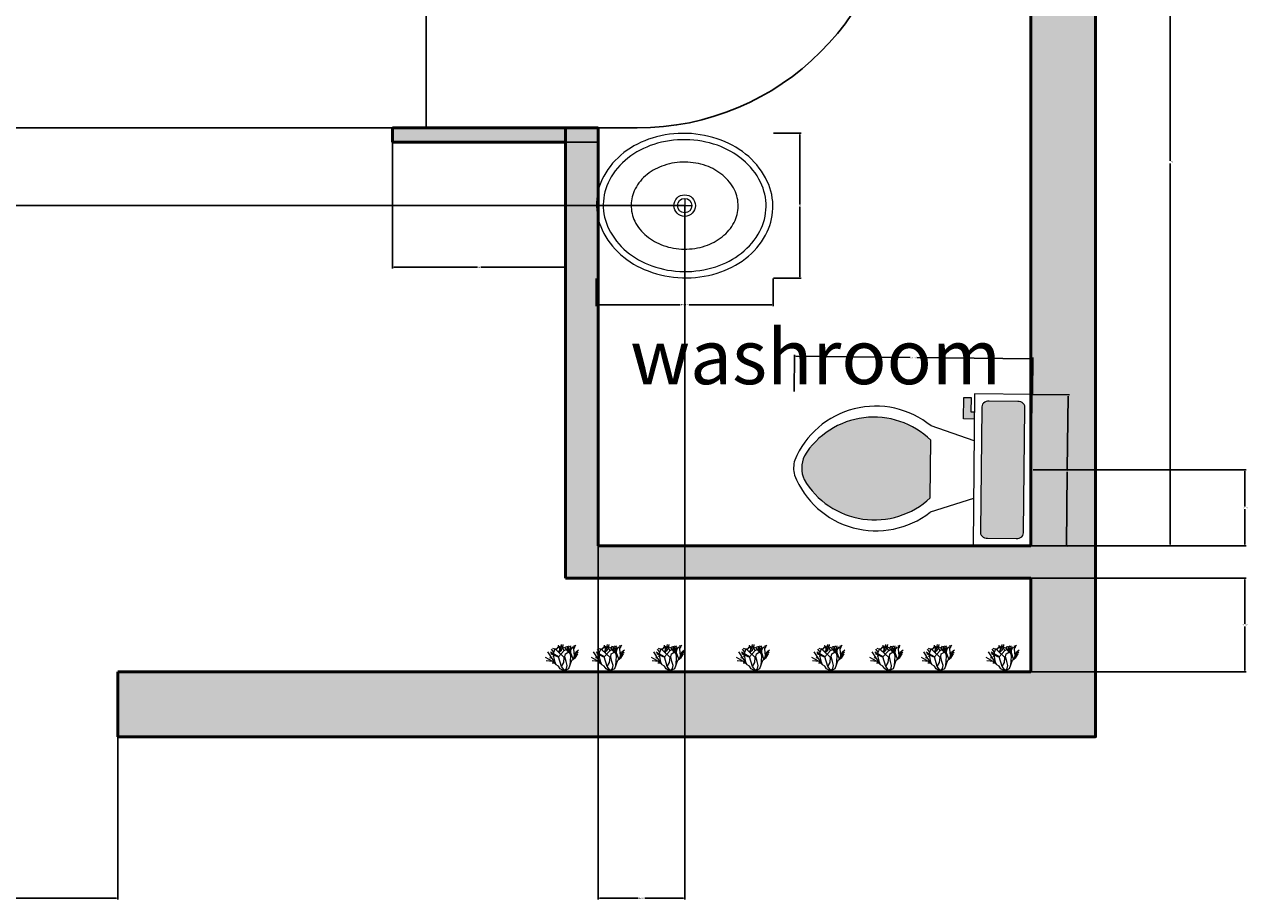
# Model space of a CAD drawing. Units: inches. Extents: x 2578 to 2919, y 51 to 451.
# Tile 3 of 5: x 2750 to 2919, y 51 to 172. Entities that reach past the tile are written whole.
import ezdxf

# ---------------------------------------------------------------- set-up
doc = ezdxf.new("R2010")
doc.units = ezdxf.units.IN
for name, color, linetype, lineweight in [('A-ANNO-DIMS', 2, 'Continuous', 18), ('A-AREA-IDEN', 7, 'Continuous', 25), ('A-DOOR', 4, 'Continuous', 25), ('A-FLOR-FIXT', 9, 'Continuous', 18), ('A-FURN-PATT', 253, 'Continuous', 13), ('A-WALL', 7, 'Continuous', 50), ('A-WALL-PATT', 250, 'Continuous', 13), ('L-PLNT', 94, 'Continuous', 13)]:
    doc.layers.add(name, color=color, linetype=linetype, lineweight=lineweight)
doc.layers.add('A-DOOR-PATT', color=29, linetype='Continuous', lineweight=13, true_color=0x4f342a)
doc.styles.get("Standard").update_dxf_attribs({"font": 'arial.ttf'})
doc.dimstyles.get("Standard").update_dxf_attribs({"dimtxt": 0.18, "dimasz": 0.18, "dimexe": 0.18, "dimexo": 0.0625, "dimgap": 0.09, "dimtad": 0, "dimtih": 1, "dimtoh": 1, "dimdec": 4, "dimzin": 0, "dimdsep": 46, "dimtxsty": 'Standard', "dimcen": 0.09, "dimadec": 0, "dimazin": 0, "dimtfac": 1, "dimtdec": 4, "dimtofl": 0, "dimtmove": 0, "dimatfit": 3, "dimfxl": 1, "dimtolj": 1, "dimtzin": 0, "dimarcsym": 0})

# ---------------------------------------------------------------- blocks, each defined once
blk = doc.blocks.new('*U3')
for p, q in [((0, 0), (0, -6)), ((40, 0), (40, -6))]:
    blk.add_line(p, q)
blk.add_lwpolyline([(0, 0), (0, 40), (1.75, 40), (1.75, 0)], close=True)
blk.add_arc((0, 0), 40, 0, 90)
blk = doc.blocks.new('Toilet - top')
for p, q in [((9.5, -6), (9.5, -2)), ((-8, -8.5), (-8, -8)), ((-7, -8), (-7, -9.5)), ((-4, -8), (-6, -14)), ((4, -8), (6, -14)), ((-10, -8.5), (-8, -8.5)), ((-10, -9.5), (-10, -8.5)), ((-7, -9.5), (-10, -9.5)), ((4, -14), (-4, -14))]:
    blk.add_line(p, q)
blk.add_lwpolyline([(10.5, -8), (10.5, 0), (-10.5, 0), (-10.5, -8)], close=True)
for points in [[(8.5, -1), (-8.5, -1)], [(-9.5, -2), (-9.5, -6)], [(-8.5, -7), (8.5, -7)]]:
    blk.add_lwpolyline(points)
for centre, radius, start, end in [((-8.62, -1.88), 0.884, 81.8699, 188.1301), ((8.62, -1.88), 0.884, 351.8699, 98.1301), ((-8.62, -6.12), 0.884, 171.8699, 278.1301), ((8.62, -6.12), 0.884, 261.8699, 8.1301), ((3.52, -21.58), 12.17, 141.4691, 247.9714), ((4.2, -21.82), 11.33, 136.3677, 238.9468), ((-3.52, -21.58), 12.17, 292.0284, 38.5307), ((-4.2, -21.82), 11.33, 301.053, 43.6321), ((0, -27.88), 4, 245.7318, 294.2682), ((0, -29), 4, 254.8605, 285.1395)]:
    blk.add_arc(centre, radius, start, end)
blk = doc.blocks.new('Sink - Oval top')
for p, q in [((-1, 0), (1, 0)), ((0, 1), (0, -1))]:
    blk.add_line(p, q)
for points in [[(-12.23, 0.39, 0.117634), (-11.46, -3.36, 0.104469), (-8.88, -6.8, 0.090016), (-5.08, -9.07, 0.08192), (-0.32, -10.02, 0.08192), (4.49, -9.38, 0.090016), (8.42, -7.36, 0.104469), (11.22, -4.09, 0.117634), (12.23, -0.39, 0.117634), (11.46, 3.36, 0.104469), (8.88, 6.8, 0.090016), (5.08, 9.07, 0.08192), (0.32, 10.02, 0.08192), (-4.49, 9.38, 0.090016), (-8.42, 7.36, 0.104469), (-11.22, 4.09, 0.117634)], [(-11.29, 0.16, 0.118622), (-10.52, -3.25, 0.104678), (-8.07, -6.36, 0.089562), (-4.54, -8.37, 0.081185), (-0.13, -9.15, 0.081185), (4.3, -8.49, 0.089562), (7.89, -6.58, 0.104678), (10.42, -3.55, 0.118622), (11.29, -0.16, 0.118622), (10.52, 3.25, 0.104678), (8.07, 6.36, 0.089562), (4.54, 8.37, 0.081185), (0.13, 9.15, 0.081185), (-4.3, 8.49, 0.089562), (-7.89, 6.58, 0.104678), (-10.42, 3.55, 0.118622)], [(-7.42, 0.08, 0.118283), (-6.91, -2.17, 0.104607), (-5.29, -4.21, 0.089718), (-2.97, -5.53, 0.081436), (-0.07, -6.04, 0.081436), (2.84, -5.59, 0.089718), (5.2, -4.33, 0.104607), (6.86, -2.32, 0.118283), (7.42, -0.08, 0.118283), (6.91, 2.17, 0.104607), (5.29, 4.21, 0.089718), (2.97, 5.53, 0.081436), (0.07, 6.04, 0.081436), (-2.84, 5.59, 0.089718), (-5.2, 4.33, 0.104607), (-6.86, 2.32, 0.118283)]]:
    blk.add_lwpolyline(points, format="xyb", close=True)
for radius in [1.5, 1]:
    blk.add_circle((0, 0), radius)
blk = doc.blocks.new('*U11')
for p, q in [((-14.88, 18.24), (-12.96, 20.64)), ((-12.471, 19.775), (-12.898, 22.044)), ((-11.28, 19.619), (-12.104, 21.184)), ((-11.921, 18.836), (-10.64, 20.401)), ((-11.433, 18.289), (-10.457, 22.749)), ((-8.16, 17.76), (-10.56, 21.6)), ((-9.48, 19.775), (-8.992, 22.592)), ((-7.2, 19.68), (-6.24, 21.12)), ((-5.086, 17.741), (-5.513, 21.34)), ((-5.28, 19.2), (-3.84, 21.6)), ((-3.84, 16.8), (-0.96, 20.64)), ((-3.377, 18.602), (-2.888, 21.575)), ((-0.508, 21.888), (-0.081, 20.558)), ((-0.203, 19.149), (0.102, 21.34)), ((-0.142, 19.384), (0.59, 20.401)), ((-0.02, 20.01), (0.896, 21.105)), ((0.041, 20.714), (1.384, 22.044)), ((0.102, 21.34), (0.835, 21.888)), ((-17.76, 8.64), (-23.663, 11.961)), ((-18.24, 11.04), (-21.755, 16.655)), ((-18.24, 11.04), (-20.16, 11.52)), ((-12.96, 12.48), (-19.68, 16.32)), ((-13.92, 12.48), (-19.2, 14.88)), ((-16.8, 16.32), (-18.72, 18.72)), ((-15.84, 8.16), (-18.24, 11.04)), ((-14.88, 18.24), (-17.76, 19.2)), ((-16.8, 12.48), (-17.76, 12.96)), ((-16.8, 16.32), (-15.36, 19.68)), ((-16.8, 12.48), (-16.8, 16.32)), ((-15.84, 8.16), (-16.8, 12.48)), ((-8.16, 12), (-14.88, 18.24)), ((-12.96, 12.48), (-13.92, 12.48)), ((-13.325, 16.724), (-11.433, 18.289)), ((-12.96, 12.48), (-8.16, 17.76)), ((-10.56, 4.32), (-12.96, 12.48)), ((-11.677, 19.071), (-12.471, 19.775)), ((-12.043, 15.628), (-11.921, 18.836)), ((-11.982, 16.802), (-10.579, 18.054)), ((-10.579, 18.054), (-9.846, 19.697)), ((-7.2, 19.68), (-8.64, 20.16)), ((-8.64, 7.68), (-8.16, 12)), ((-8.16, 17.76), (-5.28, 19.2)), ((-7.68, 12.48), (-7.2, 14.88)), ((-6.72, 8.64), (-7.68, 12.48)), ((-4.8, 16.32), (-7.2, 19.68)), ((-7.2, 14.88), (-3.84, 16.8)), ((-3.377, 15.315), (-5.086, 17.819)), ((-2.88, 12.96), (-4.32, 19.68)), ((-2.766, 16.802), (-3.377, 18.602)), ((-3.36, 5.28), (-2.88, 12.96)), ((-2.88, 15.84), (-2.4, 20.16)), ((-0.96, 10.56), (-2.88, 15.84)), ((-1.92, 9.6), (0.96, 12)), ((-0.48, 10.8), (0.346, 13.203)), ((0.346, 13.203), (-0.203, 19.149)), ((0.346, 13.203), (1.323, 16.254)), ((0.96, 12), (1.44, 15.36)), ((0.96, 12), (2.88, 14.88)), ((1.323, 16.254), (3.642, 18.289)), ((1.44, 15.36), (2.88, 17.28)), ((1.92, 13.44), (2.4, 15.36)), ((2.4, 15.36), (3.36, 16.32)), ((-17.76, 8.64), (-23.128, 9.222)), ((-16.32, 7.2), (-18.24, 7.2)), ((-14.88, 5.76), (-17.76, 8.64)), ((-15.84, 0.48), (-17.76, 0)), ((-14.88, 5.76), (-15.84, 8.16)), ((-13.44, 0.48), (-15.84, 0.48)), ((-12.96, 4.8), (-14.88, 5.76)), ((-9.6, 0.96), (-13.44, 0.48)), ((-11.52, 2.4), (-12.96, 4.8)), ((-9.6, 0.96), (-12.96, 0)), ((-8.64, 0.96), (-11.52, 2.4)), ((-10.56, 4.32), (-8.64, 7.68)), ((-8.64, 1.92), (-10.56, 4.32)), ((-9.6, 0.96), (-7.68, 0.96)), ((-8.64, 0.96), (-4.32, 2.88)), ((-8.64, 0.96), (-6.24, 2.88)), ((-8.64, 0.96), (-8.64, 1.92)), ((-8.64, 0.96), (-2.88, 0.96)), ((-7.68, 0.96), (-6.24, 0.48)), ((-5.76, 5.28), (-6.72, 8.64)), ((-6.24, 2.88), (-5.76, 5.28)), ((-6.24, 0.48), (-3.36, 0)), ((-4.32, 2.88), (-1.92, 9.6)), ((-2.88, 0.96), (0, 0))]:
    blk.add_line(p, q)
blk = doc.blocks.new('*D21')
at = {"layer": 'A-ANNO-DIMS', "color": 0, "lineweight": -2, "transparency": 16777216}
for p, q in [((2856.36, 121.01), (2856.42, 126.09)), ((2856.59, 125.9), (2872.47, 125.74)), ((2889.28, 125.56), (2873.4, 125.73)), ((2889.41, 120.66), (2889.46, 125.73))]:
    blk.add_line(p, q, dxfattribs=at)
at = {"layer": 'A-ANNO-DIMS', "color": 0, "transparency": 16777216}
for points in [[(2856.59, 125.93), (2856.59, 125.87), (2856.41, 125.91)], [(2889.28, 125.59), (2889.28, 125.53), (2889.46, 125.55)]]:
    blk.add_solid(points, dxfattribs=at)
at = {"layer": 'Defpoints', "color": 0, "transparency": 16777216}
for p in [(2889.46, 125.55), (2856.36, 120.95), (2889.41, 120.6)]:
    blk.add_point(p, dxfattribs=at)
at = {"layer": 'A-ANNO-DIMS', "color": 0, "transparency": 16777216, "insert": (2872.94, 125.73), "char_height": 0.18, "attachment_point": 5}
blk.add_mtext('\\A1;WC 33', dxfattribs=at)
blk = doc.blocks.new('*D22')
at = {"layer": 'A-ANNO-DIMS', "color": 0, "lineweight": -2, "transparency": 16777216}
for p, q in [((2889.47, 120.6), (2894.54, 120.54)), ((2894.36, 120.36), (2894.25, 110.23)), ((2894.14, 99.73), (2894.25, 109.86)), ((2889.24, 99.6), (2894.32, 99.54))]:
    blk.add_line(p, q, dxfattribs=at)
at = {"layer": 'A-ANNO-DIMS', "color": 0, "transparency": 16777216}
for points in [[(2894.33, 120.37), (2894.39, 120.36), (2894.36, 120.54)], [(2894.11, 99.73), (2894.17, 99.73), (2894.14, 99.55)]]:
    blk.add_solid(points, dxfattribs=at)
at = {"layer": 'Defpoints', "color": 0, "transparency": 16777216}
for p in [(2889.41, 120.6), (2889.18, 99.6), (2894.14, 99.55)]:
    blk.add_point(p, dxfattribs=at)
at = {"layer": 'A-ANNO-DIMS', "color": 0, "transparency": 16777216, "insert": (2894.25, 110.05), "char_height": 0.18, "attachment_point": 5}
blk.add_mtext('\\A1;21', dxfattribs=at)
blk = doc.blocks.new('*D23')
at = {"layer": 'A-ANNO-DIMS', "color": 0, "lineweight": -2, "transparency": 16777216}
for p, q in [((2828.91, 136.68), (2828.91, 132.88)), ((2853.46, 136.68), (2853.46, 132.88)), ((2829.09, 133.06), (2840.56, 133.06)), ((2853.28, 133.06), (2841.82, 133.06))]:
    blk.add_line(p, q, dxfattribs=at)
at = {"layer": 'A-ANNO-DIMS', "color": 0, "transparency": 16777216}
for points in [[(2829.09, 133.09), (2829.09, 133.03), (2828.91, 133.06)], [(2853.28, 133.09), (2853.28, 133.03), (2853.46, 133.06)]]:
    blk.add_solid(points, dxfattribs=at)
at = {"layer": 'Defpoints', "color": 0, "transparency": 16777216}
for p in [(2828.91, 136.74), (2853.46, 136.74), (2853.46, 133.06)]:
    blk.add_point(p, dxfattribs=at)
at = {"layer": 'A-ANNO-DIMS', "color": 0, "transparency": 16777216, "insert": (2841.19, 133.06), "char_height": 0.18, "attachment_point": 5}
blk.add_mtext('\\A1;BASIN 25', dxfattribs=at)
blk = doc.blocks.new('*D24')
at = {"layer": 'A-ANNO-DIMS', "color": 0, "lineweight": -2, "transparency": 16777216}
for p, q in [((2853.53, 156.88), (2857.33, 156.88)), ((2857.15, 156.7), (2857.15, 146.99)), ((2857.15, 136.92), (2857.15, 146.63)), ((2853.53, 136.74), (2857.33, 136.74))]:
    blk.add_line(p, q, dxfattribs=at)
at = {"layer": 'A-ANNO-DIMS', "color": 0, "transparency": 16777216}
for points in [[(2857.12, 156.7), (2857.18, 156.7), (2857.15, 156.88)], [(2857.12, 136.92), (2857.18, 136.92), (2857.15, 136.74)]]:
    blk.add_solid(points, dxfattribs=at)
at = {"layer": 'Defpoints', "color": 0, "transparency": 16777216}
for p in [(2853.46, 156.88), (2857.15, 156.88), (2853.46, 136.74)]:
    blk.add_point(p, dxfattribs=at)
at = {"layer": 'A-ANNO-DIMS', "color": 0, "transparency": 16777216, "insert": (2857.15, 146.81), "char_height": 0.18, "attachment_point": 5}
blk.add_mtext('\\A1;20', dxfattribs=at)
blk = doc.blocks.new('*D47')
at = {"layer": 'A-ANNO-DIMS', "color": 0, "lineweight": -2, "transparency": 16777216}
for p, q in [((2889.24, 206.11), (2908.71, 206.11)), ((2908.53, 205.93), (2908.53, 153.04)), ((2908.53, 99.78), (2908.53, 152.67)), ((2889.24, 99.6), (2908.71, 99.6))]:
    blk.add_line(p, q, dxfattribs=at)
at = {"layer": 'A-ANNO-DIMS', "color": 0, "transparency": 16777216}
for points in [[(2908.5, 205.93), (2908.56, 205.93), (2908.53, 206.11)], [(2908.5, 99.78), (2908.56, 99.78), (2908.53, 99.6)]]:
    blk.add_solid(points, dxfattribs=at)
at = {"layer": 'Defpoints', "color": 0, "transparency": 16777216}
for p in [(2889.18, 206.11), (2889.18, 99.6), (2908.53, 99.6)]:
    blk.add_point(p, dxfattribs=at)
at = {"layer": 'A-ANNO-DIMS', "color": 0, "transparency": 16777216, "insert": (2908.53, 152.85), "char_height": 0.18, "attachment_point": 5}
blk.add_mtext('\\A1;106.51', dxfattribs=at)
blk = doc.blocks.new('*D48')
at = {"layer": 'A-ANNO-DIMS', "color": 0, "lineweight": -2, "transparency": 16777216}
for p, q in [((2889.24, 95.1), (2919.06, 95.1)), ((2918.88, 94.92), (2918.88, 88.78)), ((2918.88, 82.28), (2918.88, 88.42)), ((2889.24, 82.1), (2919.06, 82.1))]:
    blk.add_line(p, q, dxfattribs=at)
at = {"layer": 'A-ANNO-DIMS', "color": 0, "transparency": 16777216}
for points in [[(2918.85, 94.92), (2918.91, 94.92), (2918.88, 95.1)], [(2918.85, 82.28), (2918.91, 82.28), (2918.88, 82.1)]]:
    blk.add_solid(points, dxfattribs=at)
at = {"layer": 'Defpoints', "color": 0, "transparency": 16777216}
for p in [(2889.18, 95.1), (2918.88, 95.1), (2889.18, 82.1)]:
    blk.add_point(p, dxfattribs=at)
at = {"layer": 'A-ANNO-DIMS', "color": 0, "transparency": 16777216, "insert": (2918.88, 88.6), "char_height": 0.18, "attachment_point": 5}
blk.add_mtext('\\A1;12.997', dxfattribs=at)
blk = doc.blocks.new('*D51')
at = {"layer": 'A-ANNO-DIMS', "color": 0, "lineweight": -2, "transparency": 16777216}
for p, q in [((2726.55, 73.04), (2726.55, 50.5)), ((2762.55, 73.04), (2762.55, 50.5)), ((2726.73, 50.68), (2744.33, 50.68)), ((2762.37, 50.68), (2744.77, 50.68))]:
    blk.add_line(p, q, dxfattribs=at)
at = {"layer": 'A-ANNO-DIMS', "color": 0, "transparency": 16777216}
for points in [[(2726.73, 50.71), (2726.73, 50.65), (2726.55, 50.68)], [(2762.37, 50.71), (2762.37, 50.65), (2762.55, 50.68)]]:
    blk.add_solid(points, dxfattribs=at)
at = {"layer": 'Defpoints', "color": 0, "transparency": 16777216}
for p in [(2726.55, 73.1), (2762.55, 73.1), (2762.55, 50.68)]:
    blk.add_point(p, dxfattribs=at)
at = {"layer": 'A-ANNO-DIMS', "color": 0, "transparency": 16777216, "insert": (2744.55, 50.68), "char_height": 0.18, "attachment_point": 5}
blk.add_mtext('\\A1;36', dxfattribs=at)
blk = doc.blocks.new('*D57')
at = {"layer": 'A-ANNO-DIMS', "color": 0, "lineweight": -2, "transparency": 16777216}
for p, q in [((2824.62, 193.6), (2805.15, 193.6)), ((2805.33, 193.42), (2805.33, 175.78)), ((2805.33, 157.78), (2805.33, 175.42)), ((2824.62, 157.6), (2805.15, 157.6))]:
    blk.add_line(p, q, dxfattribs=at)
at = {"layer": 'A-ANNO-DIMS', "color": 0, "transparency": 16777216}
for points in [[(2805.3, 193.42), (2805.36, 193.42), (2805.33, 193.6)], [(2805.3, 157.78), (2805.36, 157.78), (2805.33, 157.6)]]:
    blk.add_solid(points, dxfattribs=at)
at = {"layer": 'Defpoints', "color": 0, "transparency": 16777216}
for p in [(2805.33, 193.6), (2824.68, 193.6), (2824.68, 157.6)]:
    blk.add_point(p, dxfattribs=at)
at = {"layer": 'A-ANNO-DIMS', "color": 0, "transparency": 16777216, "insert": (2805.33, 175.6), "char_height": 0.18, "attachment_point": 5}
blk.add_mtext('\\A1;36', dxfattribs=at)
blk = doc.blocks.new('*D66')
at = {"layer": 'A-ANNO-DIMS', "color": 0, "lineweight": -2, "transparency": 16777216}
for p, q in [((2829.18, 157.54), (2829.18, 50.5)), ((2841.19, 146.75), (2841.19, 50.5)), ((2829.36, 50.68), (2834.73, 50.68)), ((2841.01, 50.68), (2835.64, 50.68))]:
    blk.add_line(p, q, dxfattribs=at)
at = {"layer": 'A-ANNO-DIMS', "color": 0, "transparency": 16777216}
for points in [[(2829.36, 50.71), (2829.36, 50.65), (2829.18, 50.68)], [(2841.01, 50.71), (2841.01, 50.65), (2841.19, 50.68)]]:
    blk.add_solid(points, dxfattribs=at)
at = {"layer": 'Defpoints', "color": 0, "transparency": 16777216}
for p in [(2829.18, 157.6), (2841.19, 146.81), (2841.19, 50.68)]:
    blk.add_point(p, dxfattribs=at)
at = {"layer": 'A-ANNO-DIMS', "color": 0, "transparency": 16777216, "insert": (2835.18, 50.68), "char_height": 0.18, "attachment_point": 5}
blk.add_mtext('\\A1;12.007', dxfattribs=at)
blk = doc.blocks.new('*D67')
at = {"layer": 'A-ANNO-DIMS', "color": 0, "lineweight": -2, "transparency": 16777216}
for p, q in [((2829.12, 157.6), (2578.02, 157.6)), ((2578.2, 157.42), (2578.2, 152.39)), ((2578.2, 146.99), (2578.2, 152.02)), ((2841.13, 146.81), (2578.02, 146.81))]:
    blk.add_line(p, q, dxfattribs=at)
at = {"layer": 'A-ANNO-DIMS', "color": 0, "transparency": 16777216}
for points in [[(2578.17, 157.42), (2578.23, 157.42), (2578.2, 157.6)], [(2578.17, 146.99), (2578.23, 146.99), (2578.2, 146.81)]]:
    blk.add_solid(points, dxfattribs=at)
at = {"layer": 'Defpoints', "color": 0, "transparency": 16777216}
for p in [(2578.2, 157.6), (2829.18, 157.6), (2841.19, 146.81)]:
    blk.add_point(p, dxfattribs=at)
at = {"layer": 'A-ANNO-DIMS', "color": 0, "transparency": 16777216, "insert": (2578.2, 152.21), "char_height": 0.18, "attachment_point": 5}
blk.add_mtext('\\A1;10.788', dxfattribs=at)
blk = doc.blocks.new('*D68')
at = {"layer": 'A-ANNO-DIMS', "color": 0, "lineweight": -2, "transparency": 16777216}
for p, q in [((2889.51, 110.13), (2919.06, 110.13)), ((2918.88, 109.95), (2918.88, 105.05)), ((2918.88, 99.78), (2918.88, 104.68)), ((2889.24, 99.6), (2919.06, 99.6))]:
    blk.add_line(p, q, dxfattribs=at)
at = {"layer": 'A-ANNO-DIMS', "color": 0, "transparency": 16777216}
for points in [[(2918.85, 109.95), (2918.91, 109.95), (2918.88, 110.13)], [(2918.85, 99.78), (2918.91, 99.78), (2918.88, 99.6)]]:
    blk.add_solid(points, dxfattribs=at)
at = {"layer": 'Defpoints', "color": 0, "transparency": 16777216}
for p in [(2889.45, 110.13), (2918.88, 110.13), (2889.18, 99.6)]:
    blk.add_point(p, dxfattribs=at)
at = {"layer": 'A-ANNO-DIMS', "color": 0, "transparency": 16777216, "insert": (2918.88, 104.87), "char_height": 0.18, "attachment_point": 5}
blk.add_mtext('\\A1;10.534', dxfattribs=at)
blk = doc.blocks.new('*D71')
at = {"layer": 'A-ANNO-DIMS', "color": 0, "lineweight": -2, "transparency": 16777216}
for p, q in [((2800.68, 157.54), (2800.68, 138.07)), ((2824.68, 157.54), (2824.68, 138.07)), ((2800.86, 138.25), (2812.46, 138.25)), ((2824.5, 138.25), (2812.9, 138.25))]:
    blk.add_line(p, q, dxfattribs=at)
at = {"layer": 'A-ANNO-DIMS', "color": 0, "transparency": 16777216}
for points in [[(2800.86, 138.28), (2800.86, 138.22), (2800.68, 138.25)], [(2824.5, 138.28), (2824.5, 138.22), (2824.68, 138.25)]]:
    blk.add_solid(points, dxfattribs=at)
at = {"layer": 'Defpoints', "color": 0, "transparency": 16777216}
for p in [(2800.68, 157.6), (2824.68, 157.6), (2800.68, 138.25)]:
    blk.add_point(p, dxfattribs=at)
at = {"layer": 'A-ANNO-DIMS', "color": 0, "transparency": 16777216, "insert": (2812.68, 138.25), "char_height": 0.18, "attachment_point": 5}
blk.add_mtext('\\A1;24', dxfattribs=at)

msp = doc.modelspace()

# ---------------------------------------------------------------- hatches: boundary and pattern name
at = {"layer": 'A-DOOR-PATT'}
h = msp.add_hatch(color=256, dxfattribs=at)
h.dxf.hatch_style = 1
h.paths.add_polyline_path([(2717.5545, 331.5492, 0.01094143), (2715.9791, 331.5147), (2715.9791, 295.5417), (2717.5545, 295.5417)])
h.paths.add_polyline_path([(2772.7563, 343.5147, 0.01094143), (2771.181, 343.5492), (2771.181, 307.5417), (2772.7563, 307.5417)])
h.paths.add_polyline_path([(2809.181, 302.1406), (2807.181, 302.1406), (2807.181, 297.6406), (2809.181, 297.6406)])
h.paths.add_polyline_path([(2681.547, 290.1406), (2679.547, 290.1406), (2679.547, 285.6406), (2681.547, 285.6406)])
h.paths.add_polyline_path([(2870.5896, 193.5988), (2834.5821, 193.5988), (2834.5821, 192.0235), (2870.5551, 192.0235, 0.01094143)])
h.paths.add_polyline_path([(2829.181, 157.5988), (2824.681, 157.5988), (2824.681, 155.5988), (2829.181, 155.5988)])
h.paths.add_polyline_path([(2702.547, 145.6406), (2698.047, 145.6406), (2698.047, 143.6481), (2702.547, 143.6481)])
h.paths.add_polyline_path([(2697.1459, 109.2159), (2661.1384, 109.2159), (2661.1384, 107.6406), (2697.1459, 107.6406)])
h.paths.add_polyline_path([(2702.547, 107.6406), (2698.047, 107.6406), (2698.047, 105.6406), (2702.547, 105.6406)])
h.paths.add_polyline_path([(2771.181, 302.1406), (2769.181, 302.1406), (2769.181, 297.6406), (2771.181, 297.6406)])
at = {"layer": 'A-FURN-PATT'}
h = msp.add_hatch(color=256, dxfattribs=at)
h.dxf.hatch_style = 1
h.paths.add_polyline_path([(2668.0284, 410.6078), (2629.3175, 410.6078), (2629.3175, 398.9331), (2619.4862, 398.9331), (2619.4862, 364.5234), (2668.0284, 364.5234)])
h.paths.add_polyline_path([(2617.6428, 398.9331), (2619.1789, 400.4692), (2619.1789, 404.4632), (2607.5042, 404.4632), (2607.5042, 388.4873), (2617.6428, 388.4873)])
h.paths.add_polyline_path([(2617.6428, 386.6439), (2607.5042, 386.6439), (2607.5042, 370.668), (2617.6428, 370.668)])
h.paths.add_polyline_path([(2875.6753, 403.5558), (2825.7487, 403.5558), (2825.7487, 356.1571), (2865.5636, 356.1571), (2865.5636, 368.1648), (2875.6753, 368.1648)])
h.paths.add_polyline_path([(2887.999, 397.2359), (2877.5713, 397.2359), (2877.5713, 380.8044), (2887.999, 380.8044)])
h.paths.add_polyline_path([(2887.999, 378.9085), (2877.5713, 378.9085), (2877.5713, 368.1648), (2875.9913, 366.5848), (2875.9913, 362.4769), (2887.999, 362.4769)])
h.paths.add_polyline_path([(2863.3609, 291.2749), (2850.0358, 291.2749), (2849.9056, 290.442), (2863.4911, 290.442)])
h.paths.add_polyline_path([(2834.6285, 271.8336), (2833.7957, 271.7035), (2833.7957, 258.3783), (2834.6285, 258.2482)])
h.paths.add_polyline_path([(2834.6285, 248.5146), (2833.7957, 248.3844), (2833.7957, 235.0593), (2834.6285, 234.9291)])
h.paths.add_polyline_path([(2879.601, 248.3844), (2878.7682, 248.5146), (2878.7682, 234.9291), (2879.601, 235.0593)])
h.paths.add_polyline_path([(2879.601, 271.7035), (2878.7682, 271.8336), (2878.7682, 258.2482), (2879.601, 258.3783)])
h.paths.add_polyline_path([(2863.4911, 216.3207), (2849.9056, 216.3207), (2850.0358, 215.4879), (2863.3609, 215.4879)])
h.paths.add_polyline_path([(2875.3365, 114.2473, 0.48007965), (2857.7894, 112.0785, 0.21500378), (2857.7543, 108.7906, 0.4800795), (2875.2511, 106.2478)])
h.paths.add_polyline_path([(2880.9002, 120.1884), (2879.9002, 120.199), (2879.8682, 117.1992), (2881.3682, 117.1832), (2881.3788, 118.1831), (2880.8789, 118.1885)])
h.paths.add_polyline_path([(2888.3838, 118.6084, 0.50000012), (2887.3945, 119.619), (2883.3947, 119.6617, 0.50000012), (2882.3841, 118.6724), (2882.2027, 101.6734, 0.50000012), (2883.192, 100.6628), (2887.1918, 100.6201, 0.50000012), (2888.2024, 101.6094)])
at = {"layer": 'A-WALL-PATT'}
h = msp.add_hatch(color=256, dxfattribs=at)
h.dxf.hatch_style = 1
h.paths.add_polyline_path([(2606.547, 422.1406), (2889.181, 422.1406), (2889.181, 210.611), (2824.681, 210.611), (2824.681, 193.5988), (2829.181, 193.5988), (2829.181, 206.111), (2889.181, 206.111), (2889.181, 99.5988), (2829.181, 99.5988), (2829.181, 155.5988), (2824.681, 155.5988), (2824.681, 95.0988), (2889.181, 95.0988), (2889.181, 82.1022), (2762.547, 82.1022), (2762.547, 73.1022), (2898.181, 73.1022), (2898.181, 233.1022), (2898.181, 431.1406), (2597.547, 431.1406), (2597.547, 73.1022), (2726.547, 73.1022), (2726.547, 82.1022), (2606.547, 82.1022), (2606.547, 173.1406), (2698.047, 173.1406), (2698.047, 145.6406), (2702.547, 145.6406), (2702.547, 157.5988), (2726.547, 157.5988), (2726.547, 177.6406), (2606.547, 177.6406)])
h.paths.add_polyline_path([(2889.181, 302.1406), (2809.181, 302.1406), (2809.181, 297.6406), (2889.181, 297.6406)], flags=17)
h.paths.add_polyline_path([(2679.547, 290.1406), (2606.547, 290.1406), (2606.547, 285.6406), (2679.547, 285.6406)], flags=17)
h.paths.add_polyline_path([(2824.681, 157.5988), (2800.681, 157.5988), (2800.681, 155.5988), (2824.681, 155.5988)], flags=17)
h.paths.add_polyline_path([(2698.047, 105.6406), (2606.547, 105.6406), (2606.547, 101.1406), (2698.047, 101.1406)], flags=17)
h.paths.add_polyline_path([(2702.547, 105.6406), (2698.047, 105.6406), (2698.047, 101.1406), (2702.547, 101.1406)], flags=17)
h.paths.add_polyline_path([(2726.547, 422.1406), (2722.047, 422.1406), (2722.047, 295.5417), (2717.5545, 295.5417), (2717.5545, 290.1406), (2717.5504, 285.6406), (2722.047, 285.6406), (2726.547, 285.6406)], flags=17)
h.paths.add_polyline_path([(2769.181, 422.1406), (2764.681, 422.1406), (2764.681, 297.6406), (2769.181, 297.6406)], flags=17)

# ---------------------------------------------------------------- linework, layer by layer
at = {"layer": 'A-DOOR'}
msp.add_line((2824.681, 155.5988), (2829.181, 155.5988), dxfattribs=at)
at = {"layer": 'A-WALL'}
for p, q in [((2889.181, 206.111), (2889.181, 99.5988)), ((2800.681, 157.5988), (2829.181, 157.5988)), ((2800.681, 157.5988), (2800.681, 155.5988)), ((2824.681, 157.5988), (2824.681, 95.0988)), ((2829.181, 157.5988), (2829.181, 99.5988)), ((2824.681, 155.5988), (2800.681, 155.5988)), ((2829.181, 99.5988), (2889.181, 99.5988)), ((2824.681, 95.0988), (2889.181, 95.0988)), ((2889.181, 95.0988), (2889.181, 82.1022)), ((2889.181, 82.1022), (2762.547, 82.1022)), ((2762.547, 73.1022), (2762.547, 82.1022)), ((2762.547, 73.1022), (2762.547, 82.1022))]:
    msp.add_line(p, q, dxfattribs=at)
msp.add_lwpolyline([(2726.547, 73.1022), (2597.547, 73.1022), (2597.547, 431.1406), (2898.181, 431.1406), (2898.181, 233.1022), (2898.181, 73.1022), (2762.547, 73.1022)], dxfattribs=at)

# ---------------------------------------------------------------- block references
at = {"layer": 'A-DOOR', "xscale": 0.9001866182309679, "yscale": 0.9001866182309679, "zscale": 0.9001866182309679, "rotation": 270}
msp.add_blockref('*U3', (2834.5821, 193.5988), dxfattribs=at)
at = {"layer": 'A-FLOR-FIXT'}
msp.add_blockref('Sink - Oval top', (2841.1879, 146.8112), dxfattribs=at)
at = {"layer": 'A-FLOR-FIXT', "rotation": 269.3886951232345}
msp.add_blockref('Toilet - top', (2889.293, 110.0982), dxfattribs=at)
at = {"layer": 'L-PLNT', "xscale": 0.1678806706863541, "yscale": 0.1678806706863541, "zscale": 0.1678806706863541}
for p in [(2825.864, 82.1022), (2832.217, 82.1022), (2840.5492, 82.1022), (2852.3499, 82.1022), (2862.8048, 82.1022), (2870.8628, 82.1022), (2877.9921, 82.1022), (2886.9781, 82.1022)]:
    msp.add_blockref('*U11', p, dxfattribs=at)

# ---------------------------------------------------------------- texts
at = {"layer": 'A-AREA-IDEN'}
msp.add_text('washroom', height=7.59312, dxfattribs=at).set_placement((2833.6234, 122.0317))

# ---------------------------------------------------------------- dimensions: what is measured, and where the dimension line sits
at = {"layer": 'A-ANNO-DIMS'}
for base, p1, p2, angle, override, picture, middle in [((2908.531, 99.5988), (2889.181, 206.111), (2889.181, 99.5988), 270, {"dimdec": 2, "dimlfac": 1, "dimrnd": 0, "dimzin": 0, "dimdsep": 46, "dimlunit": 2}, '*D47', (2908.531, 152.8549)), ((2805.331, 193.5988), (2824.681, 157.5988), (2824.681, 193.5988), 90, {"dimdec": 0, "dimlfac": 1, "dimrnd": 0, "dimzin": 0, "dimdsep": 46, "dimlunit": 2}, '*D57', (2805.331, 175.5988)), ((2578.197, 157.5988), (2841.1879, 146.8112), (2829.181, 157.5988), 90, {"dimdec": 3, "dimlfac": 1, "dimrnd": 0, "dimzin": 0, "dimdsep": 46, "dimlunit": 2}, '*D67', (2578.197, 152.205)), ((2800.681, 138.2488), (2824.681, 157.5988), (2800.681, 157.5988), 180, {"dimdec": 0, "dimlfac": 1, "dimrnd": 0, "dimzin": 0, "dimdsep": 46, "dimlunit": 2}, '*D71', (2812.681, 138.2488)), ((2857.146, 156.8795), (2853.4634, 136.7429), (2853.4634, 156.8795), 90, {"dimdec": 0, "dimlfac": 1, "dimrnd": 0, "dimzin": 0, "dimdsep": 46, "dimlunit": 2}, '*D24', (2857.146, 146.8112)), ((2894.1376, 99.546), (2889.405, 120.5977), (2889.181, 99.5988), 269.388695, {"dimdec": 0, "dimlfac": 1, "dimrnd": 0, "dimzin": 0, "dimdsep": 46, "dimlunit": 2}, '*D22', (2894.2497, 110.0454)), ((2918.8798, 110.1332), (2889.181, 99.5988), (2889.4508, 110.1332), 90, {"dimdec": 3, "dimlfac": 1, "dimrnd": 0, "dimzin": 0, "dimdsep": 46, "dimlunit": 2}, '*D68', (2918.8798, 104.866)), ((2918.8798, 95.0988), (2889.181, 82.1022), (2889.181, 95.0988), 90, {"dimdec": 3, "dimlfac": 1, "dimrnd": 0, "dimzin": 0, "dimdsep": 46, "dimlunit": 2}, '*D48', (2918.8798, 88.6005))]:
    dim = msp.add_linear_dim(base=base, p1=p1, p2=p2, angle=angle, dimstyle='Standard', override=override, dxfattribs=at)
    dim.commit()
    dim.dimension.update_dxf_attribs({"geometry": picture, "text_midpoint": middle})
for base, p1, p2, override, picture, middle in [((2841.1879, 50.6838), (2829.181, 157.5988), (2841.1879, 146.8112), {"dimdec": 3, "dimlfac": 1, "dimrnd": 0, "dimzin": 0, "dimdsep": 46, "dimlunit": 2}, '*D66', (2835.1845, 50.6838)), ((2762.547, 50.6838), (2726.547, 73.1022), (2762.547, 73.1022), {"dimdec": 0, "dimlfac": 1, "dimrnd": 0, "dimzin": 0, "dimdsep": 46, "dimlunit": 2}, '*D51', (2744.547, 50.6838))]:
    dim = msp.add_linear_dim(base=base, p1=p1, p2=p2, dimstyle='Standard', override=override, dxfattribs=at)
    dim.commit()
    dim.dimension.update_dxf_attribs({"geometry": picture, "text_midpoint": middle})
dim = msp.add_linear_dim(base=(2853.4634, 133.0602), p1=(2828.9125, 136.7429), p2=(2853.4634, 136.7429), text='BASIN <>', dimstyle='Standard', override={"dimdec": 0, "dimlfac": 1, "dimrnd": 0, "dimzin": 0, "dimdsep": 46, "dimlunit": 2}, dxfattribs=at)
dim.commit()
dim.dimension.update_dxf_attribs({"geometry": '*D23', "text_midpoint": (2841.1879, 133.0602)})
dim = msp.add_linear_dim(base=(2889.4579, 125.5543), p1=(2856.3607, 120.9502), p2=(2889.405, 120.5977), angle=359.388695, text='WC <>', dimstyle='Standard', override={"dimdec": 0, "dimlfac": 1, "dimrnd": 0, "dimzin": 0, "dimdsep": 46, "dimlunit": 2}, dxfattribs=at)
dim.commit()
dim.dimension.update_dxf_attribs({"geometry": '*D21', "text_midpoint": (2872.9357, 125.7306)})

doc.saveas('drawing.dxf')
